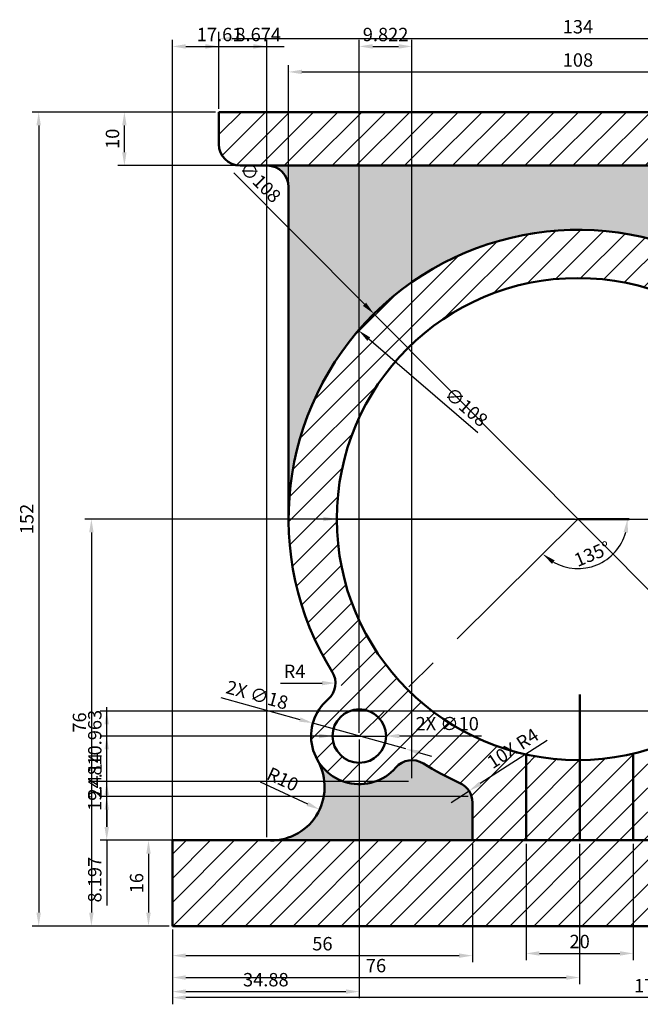
# Model space of a CAD drawing. Units: millimetres. Extents: x 2530 to 2750, y 1494 to 1677.
# Tile 1 of 2: x 2530 to 2646, y 1494 to 1677. Entities that reach past the tile are written whole.
import ezdxf

# ---------------------------------------------------------------- set-up
doc = ezdxf.new("R2010")
doc.units = ezdxf.units.MM
doc.linetypes.add('CENTER', pattern=[50.8, 31.75, -6.35, 6.35, -6.35])
for name, color, linetype, lineweight in [('M-CNTR', 1, 'CENTER', 18), ('M-DIMS', 2, 'Continuous', 25), ('M-HATC', 8, 'Continuous', 18), ('M-OUTL', 7, 'Continuous', 50)]:
    doc.layers.add(name, color=color, linetype=linetype, lineweight=lineweight)
doc.styles.get("Standard").update_dxf_attribs({"font": 'arial.ttf'})
doc.dimstyles.new('ISO-25', dxfattribs={"dimtxt": 2.5, "dimasz": 2.5, "dimexe": 1.25, "dimexo": 0.625, "dimtad": 1, "dimtxsty": 'Standard', "dimcen": 2.5, "dimadec": 0, "dimazin": 0, "dimtfac": 1, "dimtmove": 0, "dimatfit": 3, "dimfxl": 1, "dimarcsym": 0})

# ---------------------------------------------------------------- blocks, each defined once
blk = doc.blocks.new('*D1')
at = {"layer": 'Defpoints', "color": 0, "transparency": 16777216}
for p in [(2634.41, 1584.13), (2634.41, 1584.13), (2643.98, 1584.13), (2634.39, 1574.87), (2593.61, 1543.61)]:
    blk.add_point(p, dxfattribs=at)
at = {"layer": 'M-DIMS', "color": 0, "lineweight": -2, "transparency": 16777216}
blk.add_arc((2634.41, 1584.13), 9.26, 240.3168, 344.4892, dxfattribs=at)
at = {"layer": 'M-DIMS', "color": 0, "transparency": 16777216}
for points in [[(2642.92, 1581.71), (2643.75, 1581.6), (2643.67, 1584.13)], [(2629.57, 1575.75), (2630.07, 1576.41), (2627.84, 1577.6)]]:
    blk.add_solid(points, dxfattribs=at)
at = {"layer": 'M-DIMS', "color": 0, "transparency": 16777216, "insert": (2637.21, 1577.32), "char_height": 2.5, "attachment_point": 5, "rotation": 22.403}
blk.add_mtext('135°', dxfattribs=at)
blk = doc.blocks.new('*D2')
at = {"layer": 'Defpoints', "color": 0, "transparency": 16777216}
for p in [(2549.78, 1660.13), (2567.41, 1660.13), (2571.41, 1650.13)]:
    blk.add_point(p, dxfattribs=at)
at = {"layer": 'M-DIMS', "color": 0, "lineweight": -2, "transparency": 16777216}
for p, q in [((2566.78, 1660.13), (2548.53, 1660.13)), ((2549.78, 1652.63), (2549.78, 1657.63)), ((2570.78, 1650.13), (2548.53, 1650.13))]:
    blk.add_line(p, q, dxfattribs=at)
at = {"layer": 'M-DIMS', "color": 0, "transparency": 16777216}
for points in [[(2549.36, 1657.63), (2550.19, 1657.63), (2549.78, 1660.13)], [(2549.36, 1652.63), (2550.19, 1652.63), (2549.78, 1650.13)]]:
    blk.add_solid(points, dxfattribs=at)
at = {"layer": 'M-DIMS', "color": 0, "transparency": 16777216, "insert": (2547.88, 1655.13), "char_height": 2.5, "attachment_point": 5, "rotation": 90}
blk.add_mtext('10', dxfattribs=at)
blk = doc.blocks.new('*D3')
at = {"layer": 'Defpoints', "color": 0, "transparency": 16777216}
for p in [(2688.41, 1667.62), (2580.41, 1646.13), (2688.41, 1646.13)]:
    blk.add_point(p, dxfattribs=at)
at = {"layer": 'M-DIMS', "color": 0, "lineweight": -2, "transparency": 16777216}
for p, q in [((2580.41, 1646.75), (2580.41, 1668.87)), ((2688.41, 1646.75), (2688.41, 1668.87)), ((2582.91, 1667.62), (2685.91, 1667.62))]:
    blk.add_line(p, q, dxfattribs=at)
at = {"layer": 'M-DIMS', "color": 0, "transparency": 16777216}
for points in [[(2582.91, 1668.04), (2582.91, 1667.2), (2580.41, 1667.62)], [(2685.91, 1668.04), (2685.91, 1667.2), (2688.41, 1667.62)]]:
    blk.add_solid(points, dxfattribs=at)
at = {"layer": 'M-DIMS', "color": 0, "transparency": 16777216, "insert": (2634.41, 1669.52), "char_height": 2.5, "attachment_point": 5}
blk.add_mtext('108', dxfattribs=at)
blk = doc.blocks.new('*D4')
at = {"layer": 'Defpoints', "color": 0, "transparency": 16777216}
for p in [(2701.41, 1673.83), (2567.41, 1660.13), (2701.41, 1660.13)]:
    blk.add_point(p, dxfattribs=at)
at = {"layer": 'M-DIMS', "color": 0, "lineweight": -2, "transparency": 16777216}
for p, q in [((2567.41, 1660.75), (2567.41, 1675.08)), ((2701.41, 1660.75), (2701.41, 1675.08)), ((2569.91, 1673.83), (2698.91, 1673.83))]:
    blk.add_line(p, q, dxfattribs=at)
at = {"layer": 'M-DIMS', "color": 0, "transparency": 16777216}
for points in [[(2569.91, 1674.25), (2569.91, 1673.41), (2567.41, 1673.83)], [(2698.91, 1674.25), (2698.91, 1673.41), (2701.41, 1673.83)]]:
    blk.add_solid(points, dxfattribs=at)
at = {"layer": 'M-DIMS', "color": 0, "transparency": 16777216, "insert": (2634.41, 1675.73), "char_height": 2.5, "attachment_point": 5}
blk.add_mtext('134', dxfattribs=at)
blk = doc.blocks.new('*D5')
at = {"layer": 'Defpoints', "color": 0, "transparency": 16777216}
for p in [(2567.41, 1660.13), (2533.79, 1508.13), (2558.73, 1508.13)]:
    blk.add_point(p, dxfattribs=at)
at = {"layer": 'M-DIMS', "color": 0, "lineweight": -2, "transparency": 16777216}
for p, q in [((2566.78, 1660.13), (2532.54, 1660.13)), ((2533.79, 1657.63), (2533.79, 1510.63)), ((2558.11, 1508.13), (2532.54, 1508.13))]:
    blk.add_line(p, q, dxfattribs=at)
at = {"layer": 'M-DIMS', "color": 0, "transparency": 16777216}
for points in [[(2533.37, 1657.63), (2534.2, 1657.63), (2533.79, 1660.13)], [(2533.37, 1510.63), (2534.2, 1510.63), (2533.79, 1508.13)]]:
    blk.add_solid(points, dxfattribs=at)
at = {"layer": 'M-DIMS', "color": 0, "transparency": 16777216, "insert": (2531.89, 1584.13), "char_height": 2.5, "attachment_point": 5, "rotation": 90}
blk.add_mtext('152', dxfattribs=at)
blk = doc.blocks.new('*D6')
at = {"layer": 'Defpoints', "color": 0, "transparency": 16777216}
for p in [(2634.41, 1584.13), (2543.62, 1508.13), (2557.89, 1508.13)]:
    blk.add_point(p, dxfattribs=at)
at = {"layer": 'M-DIMS', "color": 0, "lineweight": -2, "transparency": 16777216}
for p, q in [((2633.78, 1584.13), (2542.37, 1584.13)), ((2543.62, 1581.63), (2543.62, 1510.63)), ((2557.27, 1508.13), (2542.37, 1508.13))]:
    blk.add_line(p, q, dxfattribs=at)
at = {"layer": 'M-DIMS', "color": 0, "transparency": 16777216}
for points in [[(2543.21, 1581.63), (2544.04, 1581.63), (2543.62, 1584.13)], [(2543.21, 1510.63), (2544.04, 1510.63), (2543.62, 1508.13)]]:
    blk.add_solid(points, dxfattribs=at)
at = {"layer": 'M-DIMS', "color": 0, "transparency": 16777216, "insert": (2541.72, 1546.13), "char_height": 2.5, "attachment_point": 5, "rotation": 90}
blk.add_mtext('76', dxfattribs=at)
blk = doc.blocks.new('*D7')
at = {"layer": 'Defpoints', "color": 0, "transparency": 16777216}
for p in [(2558.73, 1524.13), (2554.28, 1508.13), (2558.73, 1508.13)]:
    blk.add_point(p, dxfattribs=at)
at = {"layer": 'M-DIMS', "color": 0, "lineweight": -2, "transparency": 16777216}
for p, q in [((2558.11, 1524.13), (2553.03, 1524.13)), ((2554.28, 1521.63), (2554.28, 1510.63)), ((2558.11, 1508.13), (2553.03, 1508.13))]:
    blk.add_line(p, q, dxfattribs=at)
at = {"layer": 'M-DIMS', "color": 0, "transparency": 16777216}
for points in [[(2553.86, 1521.63), (2554.69, 1521.63), (2554.28, 1524.13)], [(2553.86, 1510.63), (2554.69, 1510.63), (2554.28, 1508.13)]]:
    blk.add_solid(points, dxfattribs=at)
at = {"layer": 'M-DIMS', "color": 0, "transparency": 16777216, "insert": (2552.38, 1516.13), "char_height": 2.5, "attachment_point": 5, "rotation": 90}
blk.add_mtext('16', dxfattribs=at)
blk = doc.blocks.new('*D8')
at = {"layer": 'Defpoints', "color": 0, "transparency": 16777216}
for p in [(2614.73, 1524.13), (2558.73, 1508.13), (2614.73, 1502.6)]:
    blk.add_point(p, dxfattribs=at)
at = {"layer": 'M-DIMS', "color": 0, "lineweight": -2, "transparency": 16777216}
for p, q in [((2614.73, 1523.5), (2614.73, 1501.35)), ((2558.73, 1507.5), (2558.73, 1501.35)), ((2561.23, 1502.6), (2612.23, 1502.6))]:
    blk.add_line(p, q, dxfattribs=at)
at = {"layer": 'M-DIMS', "color": 0, "transparency": 16777216}
for points in [[(2561.23, 1503.01), (2561.23, 1502.18), (2558.73, 1502.6)], [(2612.23, 1503.01), (2612.23, 1502.18), (2614.73, 1502.6)]]:
    blk.add_solid(points, dxfattribs=at)
at = {"layer": 'M-DIMS', "color": 0, "transparency": 16777216, "insert": (2586.73, 1504.5), "char_height": 2.5, "attachment_point": 5}
blk.add_mtext('56', dxfattribs=at)
blk = doc.blocks.new('*D9')
at = {"layer": 'Defpoints', "color": 0, "transparency": 16777216}
for p in [(2634.73, 1524.13), (2558.73, 1508.13), (2634.73, 1498.51)]:
    blk.add_point(p, dxfattribs=at)
at = {"layer": 'M-DIMS', "color": 0, "lineweight": -2, "transparency": 16777216}
for p, q in [((2634.73, 1523.5), (2634.73, 1497.26)), ((2558.73, 1507.5), (2558.73, 1497.26)), ((2561.23, 1498.51), (2632.23, 1498.51))]:
    blk.add_line(p, q, dxfattribs=at)
at = {"layer": 'M-DIMS', "color": 0, "transparency": 16777216}
for points in [[(2561.23, 1498.92), (2561.23, 1498.09), (2558.73, 1498.51)], [(2632.23, 1498.92), (2632.23, 1498.09), (2634.73, 1498.51)]]:
    blk.add_solid(points, dxfattribs=at)
at = {"layer": 'M-DIMS', "color": 0, "transparency": 16777216, "insert": (2596.73, 1500.41), "char_height": 2.5, "attachment_point": 5}
blk.add_mtext('76', dxfattribs=at)
blk = doc.blocks.new('*D10')
at = {"layer": 'Defpoints', "color": 0, "transparency": 16777216}
for p in [(2624.73, 1524.13), (2644.73, 1524.13), (2644.73, 1503.01)]:
    blk.add_point(p, dxfattribs=at)
at = {"layer": 'M-DIMS', "color": 0, "lineweight": -2, "transparency": 16777216}
for p, q in [((2624.73, 1523.5), (2624.73, 1501.76)), ((2644.73, 1523.5), (2644.73, 1501.76)), ((2627.23, 1503.01), (2642.23, 1503.01))]:
    blk.add_line(p, q, dxfattribs=at)
at = {"layer": 'M-DIMS', "color": 0, "transparency": 16777216}
for points in [[(2627.23, 1503.43), (2627.23, 1502.59), (2624.73, 1503.01)], [(2642.23, 1503.43), (2642.23, 1502.59), (2644.73, 1503.01)]]:
    blk.add_solid(points, dxfattribs=at)
at = {"layer": 'M-DIMS', "color": 0, "transparency": 16777216, "insert": (2634.73, 1504.91), "char_height": 2.5, "attachment_point": 5}
blk.add_mtext('20', dxfattribs=at)
blk = doc.blocks.new('*D14')
at = {"layer": 'Defpoints', "color": 0, "transparency": 16777216}
for p in [(2558.73, 1508.13), (2736.73, 1508.13), (2558.73, 1494.76)]:
    blk.add_point(p, dxfattribs=at)
at = {"layer": 'M-DIMS', "color": 0, "lineweight": -2, "transparency": 16777216}
for p, q in [((2558.73, 1507.5), (2558.73, 1493.51)), ((2736.73, 1507.5), (2736.73, 1493.51)), ((2734.23, 1494.76), (2561.23, 1494.76))]:
    blk.add_line(p, q, dxfattribs=at)
at = {"layer": 'M-DIMS', "color": 0, "transparency": 16777216}
for points in [[(2561.23, 1495.17), (2561.23, 1494.34), (2558.73, 1494.76)], [(2734.23, 1495.17), (2734.23, 1494.34), (2736.73, 1494.76)]]:
    blk.add_solid(points, dxfattribs=at)
at = {"layer": 'M-DIMS', "color": 0, "transparency": 16777216, "insert": (2647.73, 1496.66), "char_height": 2.5, "attachment_point": 5}
blk.add_mtext('178', dxfattribs=at)
blk = doc.blocks.new('*D17')
at = {"layer": 'Defpoints', "color": 0, "transparency": 16777216}
for p in [(2577.14, 1534.1), (2586.2, 1529.88)]:
    blk.add_point(p, dxfattribs=at)
at = {"layer": 'M-DIMS', "color": 0, "lineweight": -2, "transparency": 16777216}
blk.add_line((2575.13, 1535.03), (2583.94, 1530.94), dxfattribs=at)
at = {"layer": 'M-DIMS', "color": 0, "transparency": 16777216}
blk.add_solid([(2584.11, 1531.31), (2583.76, 1530.56), (2586.2, 1529.88)], dxfattribs=at)
at = {"layer": 'M-DIMS', "color": 0, "transparency": 16777216, "insert": (2579.2, 1535.24), "char_height": 2.5, "attachment_point": 5, "rotation": 335.0749}
blk.add_mtext('R10', dxfattribs=at)
blk = doc.blocks.new('*D24')
at = {"layer": 'Defpoints', "color": 0, "transparency": 16777216}
for p in [(2585.16, 1553.49), (2589.16, 1553.49)]:
    blk.add_point(p, dxfattribs=at)
at = {"layer": 'M-DIMS', "color": 0, "lineweight": -2, "transparency": 16777216}
blk.add_line((2578.89, 1553.49), (2586.66, 1553.49), dxfattribs=at)
at = {"layer": 'M-DIMS', "color": 0, "transparency": 16777216}
blk.add_solid([(2586.66, 1553.9), (2586.66, 1553.07), (2589.16, 1553.49)], dxfattribs=at)
at = {"layer": 'M-DIMS', "color": 0, "transparency": 16777216, "insert": (2581.53, 1555.36), "char_height": 2.5, "attachment_point": 5}
blk.add_mtext('R4', dxfattribs=at)
blk = doc.blocks.new('*D25')
at = {"layer": 'Defpoints', "color": 0, "transparency": 16777216}
for p in [(2672.67, 1607.82), (2596.15, 1560.44)]:
    blk.add_point(p, dxfattribs=at)
at = {"layer": 'M-DIMS', "color": 0, "lineweight": -2, "transparency": 16777216}
blk.add_line((2662, 1601.22), (2670.54, 1606.5), dxfattribs=at)
at = {"layer": 'M-DIMS', "color": 0, "transparency": 16777216}
blk.add_solid([(2670.32, 1606.86), (2670.76, 1606.15), (2672.67, 1607.82)], dxfattribs=at)
at = {"layer": 'M-DIMS', "color": 0, "transparency": 16777216, "insert": (2664.17, 1604.88), "char_height": 2.5, "attachment_point": 5, "rotation": 31.768}
blk.add_mtext('∅90', dxfattribs=at)
blk = doc.blocks.new('*D26')
at = {"layer": 'Defpoints', "color": 0, "transparency": 16777216}
for p in [(2593.48, 1619.36), (2675.33, 1548.9)]:
    blk.add_point(p, dxfattribs=at)
at = {"layer": 'M-DIMS', "color": 0, "lineweight": -2, "transparency": 16777216}
blk.add_line((2615.7, 1600.23), (2595.38, 1617.73), dxfattribs=at)
at = {"layer": 'M-DIMS', "color": 0, "transparency": 16777216}
blk.add_solid([(2595.65, 1618.04), (2595.11, 1617.41), (2593.48, 1619.36)], dxfattribs=at)
at = {"layer": 'M-DIMS', "color": 0, "transparency": 16777216, "insert": (2613.39, 1604.82), "char_height": 2.5, "attachment_point": 5, "rotation": 319.2753}
blk.add_mtext('∅108', dxfattribs=at)
blk = doc.blocks.new('*D27')
at = {"layer": 'Defpoints', "color": 0, "transparency": 16777216}
for p in [(2593.61, 1543.61), (2558.73, 1508.13), (2593.61, 1495.88)]:
    blk.add_point(p, dxfattribs=at)
at = {"layer": 'M-DIMS', "color": 0, "lineweight": -2, "transparency": 16777216}
for p, q in [((2593.61, 1542.98), (2593.61, 1494.63)), ((2558.73, 1507.5), (2558.73, 1494.63)), ((2561.23, 1495.88), (2591.11, 1495.88))]:
    blk.add_line(p, q, dxfattribs=at)
at = {"layer": 'M-DIMS', "color": 0, "transparency": 16777216}
for points in [[(2561.23, 1496.3), (2561.23, 1495.46), (2558.73, 1495.88)], [(2591.11, 1496.3), (2591.11, 1495.46), (2593.61, 1495.88)]]:
    blk.add_solid(points, dxfattribs=at)
at = {"layer": 'M-DIMS', "color": 0, "transparency": 16777216, "insert": (2576.17, 1497.78), "char_height": 2.5, "attachment_point": 5}
blk.add_mtext('34.88', dxfattribs=at)
blk = doc.blocks.new('*D28')
at = {"layer": 'Defpoints', "color": 0, "transparency": 16777216}
for p in [(2546.48, 1543.61), (2593.61, 1543.61), (2576.34, 1524.13)]:
    blk.add_point(p, dxfattribs=at)
at = {"layer": 'M-DIMS', "color": 0, "lineweight": -2, "transparency": 16777216}
for p, q in [((2592.99, 1543.61), (2545.23, 1543.61)), ((2546.48, 1526.63), (2546.48, 1541.11)), ((2575.72, 1524.13), (2545.23, 1524.13))]:
    blk.add_line(p, q, dxfattribs=at)
at = {"layer": 'M-DIMS', "color": 0, "transparency": 16777216}
for points in [[(2546.07, 1541.11), (2546.9, 1541.11), (2546.48, 1543.61)], [(2546.07, 1526.63), (2546.9, 1526.63), (2546.48, 1524.13)]]:
    blk.add_solid(points, dxfattribs=at)
at = {"layer": 'M-DIMS', "color": 0, "transparency": 16777216, "insert": (2544.58, 1533.87), "char_height": 2.5, "attachment_point": 5, "rotation": 90}
blk.add_mtext('19.48', dxfattribs=at)
blk = doc.blocks.new('*D31')
at = {"layer": 'Defpoints', "color": 0, "transparency": 16777216}
for p in [(2614.57, 1532.33), (2546.48, 1524.13), (2614.73, 1524.13)]:
    blk.add_point(p, dxfattribs=at)
at = {"layer": 'M-DIMS', "color": 0, "lineweight": -2, "transparency": 16777216}
for p, q in [((2613.94, 1532.33), (2545.23, 1532.33)), ((2546.48, 1529.83), (2546.48, 1526.63)), ((2614.11, 1524.13), (2545.23, 1524.13)), ((2546.48, 1524.13), (2546.48, 1511.94))]:
    blk.add_line(p, q, dxfattribs=at)
at = {"layer": 'M-DIMS', "color": 0, "transparency": 16777216}
for points in [[(2546.07, 1529.83), (2546.9, 1529.83), (2546.48, 1532.33)], [(2546.07, 1526.63), (2546.9, 1526.63), (2546.48, 1524.13)]]:
    blk.add_solid(points, dxfattribs=at)
at = {"layer": 'M-DIMS', "color": 0, "transparency": 16777216, "insert": (2544.58, 1516.78), "char_height": 2.5, "attachment_point": 5, "rotation": 90}
blk.add_mtext('8.197', dxfattribs=at)
blk = doc.blocks.new('*D32')
at = {"layer": 'Defpoints', "color": 0, "transparency": 16777216}
for p in [(2576.34, 1672.38), (2558.73, 1524.13), (2576.34, 1524.13)]:
    blk.add_point(p, dxfattribs=at)
at = {"layer": 'M-DIMS', "color": 0, "lineweight": -2, "transparency": 16777216}
for p, q in [((2558.73, 1524.75), (2558.73, 1673.63)), ((2576.34, 1524.75), (2576.34, 1673.63)), ((2561.23, 1672.38), (2573.84, 1672.38))]:
    blk.add_line(p, q, dxfattribs=at)
at = {"layer": 'M-DIMS', "color": 0, "transparency": 16777216}
for points in [[(2561.23, 1672.8), (2561.23, 1671.96), (2558.73, 1672.38)], [(2573.84, 1672.8), (2573.84, 1671.96), (2576.34, 1672.38)]]:
    blk.add_solid(points, dxfattribs=at)
at = {"layer": 'M-DIMS', "color": 0, "transparency": 16777216, "insert": (2567.54, 1674.28), "char_height": 2.5, "attachment_point": 5}
blk.add_mtext('17.61', dxfattribs=at)
blk = doc.blocks.new('*D33')
at = {"layer": 'Defpoints', "color": 0, "transparency": 16777216}
for p in [(2567.41, 1672.38), (2567.41, 1660.13), (2558.73, 1508.13)]:
    blk.add_point(p, dxfattribs=at)
at = {"layer": 'M-DIMS', "color": 0, "lineweight": -2, "transparency": 16777216}
for p, q in [((2558.73, 1508.75), (2558.73, 1673.63)), ((2567.41, 1660.75), (2567.41, 1673.63)), ((2561.23, 1672.38), (2564.91, 1672.38)), ((2567.41, 1672.38), (2579.59, 1672.38))]:
    blk.add_line(p, q, dxfattribs=at)
at = {"layer": 'M-DIMS', "color": 0, "transparency": 16777216}
for points in [[(2561.23, 1672.8), (2561.23, 1671.96), (2558.73, 1672.38)], [(2564.91, 1672.8), (2564.91, 1671.96), (2567.41, 1672.38)]]:
    blk.add_solid(points, dxfattribs=at)
at = {"layer": 'M-DIMS', "color": 0, "transparency": 16777216, "insert": (2574.75, 1674.28), "char_height": 2.5, "attachment_point": 5}
blk.add_mtext('8.674', dxfattribs=at)
blk = doc.blocks.new('*D36')
at = {"layer": 'Defpoints', "color": 0, "transparency": 16777216}
for p in [(2546.48, 1548.27), (2682.63, 1548.27), (2677.41, 1524.13)]:
    blk.add_point(p, dxfattribs=at)
at = {"layer": 'M-DIMS', "color": 0, "lineweight": -2, "transparency": 16777216}
for p, q in [((2682, 1548.27), (2545.23, 1548.27)), ((2546.48, 1526.63), (2546.48, 1545.77)), ((2676.78, 1524.13), (2545.23, 1524.13))]:
    blk.add_line(p, q, dxfattribs=at)
at = {"layer": 'M-DIMS', "color": 0, "transparency": 16777216}
for points in [[(2546.07, 1545.77), (2546.9, 1545.77), (2546.48, 1548.27)], [(2546.07, 1526.63), (2546.9, 1526.63), (2546.48, 1524.13)]]:
    blk.add_solid(points, dxfattribs=at)
at = {"layer": 'M-DIMS', "color": 0, "transparency": 16777216, "insert": (2544.6, 1536.2), "char_height": 2.5, "attachment_point": 5, "rotation": 90}
blk.add_mtext('24.14', dxfattribs=at)
blk = doc.blocks.new('*D37')
at = {"layer": 'Defpoints', "color": 0, "transparency": 16777216}
for p in [(2603.43, 1672.38), (2593.61, 1543.61), (2603.43, 1535.09)]:
    blk.add_point(p, dxfattribs=at)
at = {"layer": 'M-DIMS', "color": 0, "lineweight": -2, "transparency": 16777216}
for p, q in [((2593.61, 1544.23), (2593.61, 1673.63)), ((2603.43, 1535.72), (2603.43, 1673.63)), ((2596.11, 1672.38), (2600.93, 1672.38))]:
    blk.add_line(p, q, dxfattribs=at)
at = {"layer": 'M-DIMS', "color": 0, "transparency": 16777216}
for points in [[(2596.11, 1672.8), (2596.11, 1671.96), (2593.61, 1672.38)], [(2600.93, 1672.8), (2600.93, 1671.96), (2603.43, 1672.38)]]:
    blk.add_solid(points, dxfattribs=at)
at = {"layer": 'M-DIMS', "color": 0, "transparency": 16777216, "insert": (2598.52, 1674.28), "char_height": 2.5, "attachment_point": 5}
blk.add_mtext('9.822', dxfattribs=at)
blk = doc.blocks.new('*D38')
at = {"layer": 'Defpoints', "color": 0, "transparency": 16777216}
for p in [(2546.48, 1535.09), (2603.43, 1535.09), (2614.73, 1524.13)]:
    blk.add_point(p, dxfattribs=at)
at = {"layer": 'M-DIMS', "color": 0, "lineweight": -2, "transparency": 16777216}
for p, q in [((2546.48, 1535.09), (2546.48, 1548.99)), ((2602.81, 1535.09), (2545.23, 1535.09)), ((2546.48, 1526.63), (2546.48, 1532.59)), ((2614.11, 1524.13), (2545.23, 1524.13))]:
    blk.add_line(p, q, dxfattribs=at)
at = {"layer": 'M-DIMS', "color": 0, "transparency": 16777216}
for points in [[(2546.07, 1532.59), (2546.9, 1532.59), (2546.48, 1535.09)], [(2546.07, 1526.63), (2546.9, 1526.63), (2546.48, 1524.13)]]:
    blk.add_solid(points, dxfattribs=at)
at = {"layer": 'M-DIMS', "color": 0, "transparency": 16777216, "insert": (2544.58, 1543.29), "char_height": 2.5, "attachment_point": 5, "rotation": 90}
blk.add_mtext('10.963', dxfattribs=at)
blk = doc.blocks.new('*D39')
at = {"layer": 'Defpoints', "color": 0, "transparency": 16777216}
for p in [(2596.35, 1622.44), (2672.46, 1545.82)]:
    blk.add_point(p, dxfattribs=at)
at = {"layer": 'M-DIMS', "color": 0, "lineweight": -2, "transparency": 16777216}
for p, q in [((2570.17, 1648.8), (2594.59, 1624.22)), ((2672.46, 1545.82), (2596.35, 1622.44)), ((2674.22, 1544.04), (2675.99, 1542.27))]:
    blk.add_line(p, q, dxfattribs=at)
at = {"layer": 'M-DIMS', "color": 0, "transparency": 16777216}
for points in [[(2594.89, 1624.51), (2594.3, 1623.92), (2596.35, 1622.44)], [(2674.52, 1544.34), (2673.93, 1543.75), (2672.46, 1545.82)]]:
    blk.add_solid(points, dxfattribs=at)
at = {"layer": 'M-DIMS', "color": 0, "transparency": 16777216, "insert": (2574.92, 1646.82), "char_height": 2.5, "attachment_point": 5, "rotation": 314.806}
blk.add_mtext('∅108', dxfattribs=at)
blk = doc.blocks.new('*D40')
at = {"layer": 'Defpoints', "color": 0, "transparency": 16777216}
for p in [(2589.41, 1584.13), (2679.41, 1584.13)]:
    blk.add_point(p, dxfattribs=at)
at = {"layer": 'M-DIMS', "color": 0, "lineweight": -2, "transparency": 16777216}
for p, q in [((2586.91, 1584.13), (2584.41, 1584.13)), ((2589.41, 1584.13), (2679.41, 1584.13)), ((2710.18, 1584.13), (2681.91, 1584.13))]:
    blk.add_line(p, q, dxfattribs=at)
at = {"layer": 'M-DIMS', "color": 0, "transparency": 16777216}
for points in [[(2586.91, 1584.55), (2586.91, 1583.71), (2589.41, 1584.13)], [(2681.91, 1584.55), (2681.91, 1583.71), (2679.41, 1584.13)]]:
    blk.add_solid(points, dxfattribs=at)
at = {"layer": 'M-DIMS', "color": 0, "transparency": 16777216, "insert": (2706.41, 1586.1), "char_height": 2.5, "attachment_point": 5, "rotation": 0.0001}
blk.add_mtext('∅90', dxfattribs=at)
blk = doc.blocks.new('*D41')
at = {"layer": 'Defpoints', "color": 0, "transparency": 16777216}
for p in [(2584.94, 1546.02), (2602.28, 1541.2)]:
    blk.add_point(p, dxfattribs=at)
at = {"layer": 'M-DIMS', "color": 0, "lineweight": -2, "transparency": 16777216}
for p, q in [((2567.75, 1550.79), (2582.53, 1546.69)), ((2602.28, 1541.2), (2584.94, 1546.02)), ((2604.69, 1540.53), (2607.1, 1539.86))]:
    blk.add_line(p, q, dxfattribs=at)
at = {"layer": 'M-DIMS', "color": 0, "transparency": 16777216}
for points in [[(2582.64, 1547.09), (2582.42, 1546.28), (2584.94, 1546.02)], [(2604.8, 1540.93), (2604.58, 1540.13), (2602.28, 1541.2)]]:
    blk.add_solid(points, dxfattribs=at)
at = {"layer": 'M-DIMS', "color": 0, "transparency": 16777216, "insert": (2574.47, 1550.97), "char_height": 2.5, "attachment_point": 5, "rotation": 344.4794}
blk.add_mtext('2X ∅18', dxfattribs=at)
blk = doc.blocks.new('*D42')
at = {"layer": 'Defpoints', "color": 0, "transparency": 16777216}
for p in [(2588.61, 1543.61), (2598.61, 1543.61)]:
    blk.add_point(p, dxfattribs=at)
at = {"layer": 'M-DIMS', "color": 0, "lineweight": -2, "transparency": 16777216}
for p, q in [((2586.11, 1543.61), (2583.61, 1543.61)), ((2588.61, 1543.61), (2598.61, 1543.61)), ((2616.44, 1543.61), (2601.11, 1543.61))]:
    blk.add_line(p, q, dxfattribs=at)
at = {"layer": 'M-DIMS', "color": 0, "transparency": 16777216}
for points in [[(2586.11, 1544.03), (2586.11, 1543.19), (2588.61, 1543.61)], [(2601.11, 1544.02), (2601.11, 1543.19), (2598.61, 1543.61)]]:
    blk.add_solid(points, dxfattribs=at)
at = {"layer": 'M-DIMS', "color": 0, "transparency": 16777216, "insert": (2610.02, 1545.58), "char_height": 2.5, "attachment_point": 5, "rotation": 359.9972}
blk.add_mtext('2X ∅10', dxfattribs=at)
blk = doc.blocks.new('*D43')
at = {"layer": 'Defpoints', "color": 0, "transparency": 16777216}
for p in [(2614.09, 1533.36), (2610.73, 1531.18)]:
    blk.add_point(p, dxfattribs=at)
at = {"layer": 'M-DIMS', "color": 0, "lineweight": -2, "transparency": 16777216}
for p, q in [((2628.65, 1542.79), (2616.19, 1534.72)), ((2610.73, 1531.18), (2614.09, 1533.36))]:
    blk.add_line(p, q, dxfattribs=at)
at = {"layer": 'M-DIMS', "color": 0, "transparency": 16777216}
blk.add_solid([(2615.96, 1535.07), (2616.42, 1534.37), (2614.09, 1533.36)], dxfattribs=at)
at = {"layer": 'M-DIMS', "color": 0, "transparency": 16777216, "insert": (2622.43, 1541.03), "char_height": 2.5, "attachment_point": 5, "rotation": 32.9488}
blk.add_mtext('10X R4', dxfattribs=at)

msp = doc.modelspace()

# ---------------------------------------------------------------- hatches: boundary and pattern name
at = {"layer": 'M-HATC'}
h = msp.add_hatch(dxfattribs=at)
h.set_pattern_fill('ANSI31', color=256)
h.paths.add_polyline_path([(2701.4085, 1660.1289), (2688.4085, 1660.1289), (2567.4085, 1660.1289), (2567.4085, 1654.1289, 0.41421356), (2571.4085, 1650.1289), (2580.4085, 1650.1289), (2688.4085, 1650.1289), (2697.4085, 1650.1289, 0.41421356), (2701.4085, 1654.1289)])
h.paths.add_polyline_path([(2679.4085, 1584.1289, -0.34791599), (2644.7344, 1540.3297), (2644.7344, 1524.1289), (2654.7344, 1524.1289), (2658.7344, 1524.1289, -0.41421356), (2654.7344, 1528.1289), (2654.7344, 1531.4768, -0.29243225), (2657.0568, 1535.108, 0.47416598), (2677.944, 1616.0767, 1.63457651), (2666.6504, 1627.447, 0.86114512), (2590.873, 1552.1812, 1.31927608), (2600.4123, 1537.7124, -0.37066508), (2605.5707, 1538.4739, 0.03574325), (2612.3671, 1534.8321, -0.29578567), (2614.7344, 1531.1805), (2614.7344, 1524.1289), (2624.7344, 1524.1289), (2624.7344, 1540.1811, -0.14401207), (2602.4811, 1552.4171), (2597.1599, 1547.1318, -0.19803221), (2598.6124, 1543.6082, -1), (2588.6124, 1543.6082, -0.6694042), (2597.1599, 1547.1318), (2602.4811, 1552.4171, -0.19803221), (2589.4085, 1584.1289, -1)])
h.paths.add_polyline_path([(2680.2046, 1624.6496, -1), (2670.2046, 1624.6496, -1)], flags=16)
h.paths.add_polyline_path([(2736.7344, 1524.1289), (2735.977, 1524.1289, -0.04128859), (2734.3283, 1524.1289), (2577.9283, 1524.1289, -0.03968429), (2576.3434, 1524.1289), (2558.7344, 1524.1289), (2558.7344, 1508.1289), (2736.7344, 1508.1289)])
h = msp.add_hatch(color=256, dxfattribs=at)
h.dxf.hatch_style = 1
h.paths.add_polyline_path([(2688.4085, 1646.1289, -0.41421356), (2692.4085, 1650.1289), (2688.4085, 1650.1289), (2580.4085, 1650.1289), (2576.4085, 1650.1289, -0.41421356), (2580.4085, 1646.1289), (2580.4085, 1584.1289, -0.61677219), (2666.6504, 1627.447, -1.63457651), (2677.944, 1616.0767, -0.15960296), (2688.4085, 1584.1289)])
h.paths.add_polyline_path([(2696.1494, 1571.5708, -0.30814487), (2688.4024, 1583.3173, -0.28835772), (2657.0568, 1535.108, 0.29243225), (2654.7344, 1531.4768), (2654.7344, 1528.1289, 0.41421356), (2658.7344, 1524.1289), (2677.4085, 1524.1289), (2682.6254, 1548.2693, -0.35316368), (2694.8434, 1558.1289), (2696.2102, 1558.1289)])
h.paths.add_polyline_path([(2713.9085, 1558.1289, 0.30415201), (2706.158, 1569.6915), (2706.2106, 1558.0572, -0.18754445), (2709.4561, 1551.5776), (2714.9622, 1524.1289), (2734.3283, 1524.1289, -0.27714511), (2725.9689, 1530.1379)])
h.paths.add_polyline_path([(2614.7344, 1531.1805, 0.29578567), (2612.3671, 1534.8321, -0.03574325), (2605.5707, 1538.4739, 0.37066508), (2600.4123, 1537.7124, -0.512533), (2585.8599, 1539.0368), (2585.8445, 1539.0127, -0.54802528), (2577.9283, 1524.1289), (2614.7344, 1524.1289)])
h = msp.add_hatch(dxfattribs=at)
h.set_pattern_fill('ANSI31', color=256)
h.paths.add_polyline_path([(2634.7344, 1539.1301, -0.05603695), (2624.7344, 1540.1811), (2624.7344, 1524.1289), (2634.7344, 1524.1289)])
h.paths.add_polyline_path([(2644.7344, 1540.3297, -0.05613012), (2634.7344, 1539.1301), (2634.7344, 1524.1289), (2644.7344, 1524.1289)])

# ---------------------------------------------------------------- linework, layer by layer
at = {"layer": 'M-CNTR'}
msp.add_line((2634.4085, 1584.1289), (2593.6124, 1543.6082), dxfattribs=at)
at = {"layer": 'M-OUTL'}
for p, q in [((2567.4085, 1654.1289), (2567.4085, 1660.1289)), ((2567.4085, 1660.1289), (2688.4085, 1660.1289)), ((2580.4085, 1650.1289), (2571.4085, 1650.1289)), ((2580.4085, 1650.1289), (2688.4085, 1650.1289)), ((2580.4085, 1584.1289), (2580.4085, 1646.1289)), ((2634.4085, 1584.1289), (2643.9827, 1584.1289)), ((2634.7344, 1524.1289), (2634.7344, 1551.3374)), ((2585.8445, 1539.0127), (2585.8599, 1539.0368)), ((2590.5939, 1540.6102), (2590.5939, 1540.6102)), ((2624.7344, 1524.1289), (2624.7344, 1540.1811)), ((2644.7344, 1524.1289), (2644.7344, 1540.3297)), ((2614.7344, 1524.1289), (2614.7344, 1531.1805)), ((2558.7344, 1524.1289), (2736.7344, 1524.1289)), ((2558.7344, 1524.1289), (2614.7344, 1524.1289)), ((2558.7344, 1508.1289), (2558.7344, 1524.1289)), ((2614.7344, 1524.1289), (2634.7344, 1524.1289)), ((2644.7344, 1524.1289), (2654.7344, 1524.1289)), ((2558.7344, 1508.1289), (2736.7344, 1508.1289))]:
    msp.add_line(p, q, dxfattribs=at)
for centre, radius in [((2634.4085, 1584.1289), 45), ((2593.6124, 1543.6082), 5)]:
    msp.add_circle(centre, radius, dxfattribs=at)
for centre, radius, start, end in [((2571.4085, 1654.1289), 4, 180, 270), ((2576.4085, 1646.1289), 4, 0, 90), ((2634.4085, 1584.1289), 54, 57.721584, 211.89027), ((2585.1629, 1553.4879), 4, 310.538333, 31.89027), ((2593.6124, 1543.6082), 9, 130.538333, 319.073521), ((2577.1358, 1534.0975), 10, 265.4549, 29.440521), ((2603.4345, 1535.0921), 4, 57.721584, 139.073521), ((2634.4085, 1584.1289), 54, 237.721584, 245.909848), ((2610.7344, 1531.1805), 4, 360, 65.909848)]:
    msp.add_arc(centre, radius, start, end, dxfattribs=at)

# ---------------------------------------------------------------- dimensions: what is measured, and where the dimension line sits
at = {"layer": 'M-DIMS'}
for base, p1, p2, override, picture, middle in [((2701.4085, 1673.8298), (2567.4085, 1660.1289), (2701.4085, 1660.1289), {"dimclrd": 0, "dimclre": 0, "dimclrt": 0}, '*D4', (2634.4085, 1675.7321)), ((2576.3434, 1672.3789), (2558.7344, 1524.1289), (2576.3434, 1524.1289), {"dimdec": 2, "dimlfac": 1, "dimrnd": 0, "dimzin": 0, "dimdsep": 46, "dimlunit": 2}, '*D32', (2567.5389, 1674.2804)), ((2567.4085, 1672.3789), (2558.7344, 1508.1289), (2567.4085, 1660.1289), {"dimdec": 3, "dimlfac": 1, "dimrnd": 0, "dimzin": 0, "dimdsep": 46, "dimlunit": 2}, '*D33', (2574.7482, 1674.2804)), ((2603.4345, 1672.3789), (2593.6124, 1543.6082), (2603.4345, 1535.0921), {"dimdec": 3, "dimlfac": 1, "dimrnd": 0, "dimzin": 0, "dimdsep": 46, "dimlunit": 2}, '*D37', (2598.5235, 1674.2804)), ((2688.4085, 1667.6183), (2580.4085, 1646.1289), (2688.4085, 1646.1289), {"dimclrd": 0, "dimclre": 0, "dimclrt": 0}, '*D3', (2634.4085, 1669.5198)), ((2593.6124, 1495.8789), (2558.7344, 1508.1289), (2593.6124, 1543.6082), {"dimdec": 2, "dimlfac": 1, "dimrnd": 0, "dimzin": 0, "dimdsep": 46, "dimlunit": 2}, '*D27', (2576.1734, 1497.7812)), ((2614.7344, 1502.595), (2558.7344, 1508.1289), (2614.7344, 1524.1289), {"dimclrd": 0, "dimclre": 0, "dimclrt": 0}, '*D8', (2586.7344, 1504.4964)), ((2634.7344, 1498.5081), (2558.7344, 1508.1289), (2634.7344, 1524.1289), {"dimclrd": 0, "dimclre": 0, "dimclrt": 0}, '*D9', (2596.7344, 1500.4096)), ((2644.7344, 1503.0087), (2624.7344, 1524.1289), (2644.7344, 1524.1289), {"dimclrd": 0, "dimclre": 0, "dimclrt": 0}, '*D10', (2634.7344, 1504.9102)), ((2558.7344, 1494.7581), (2736.7344, 1508.1289), (2558.7344, 1508.1289), {"dimclrd": 0, "dimclre": 0, "dimclrt": 0}, '*D14', (2647.7344, 1496.6596))]:
    dim = msp.add_linear_dim(base=base, p1=p1, p2=p2, dimstyle='ISO-25', override=override, dxfattribs=at)
    dim.commit()
    dim.dimension.update_dxf_attribs({"geometry": picture, "text_midpoint": middle})
for base, p1, p2, override, picture, middle in [((2533.787, 1508.1289), (2567.4085, 1660.1289), (2558.7344, 1508.1289), {"dimclrd": 0, "dimclre": 0, "dimclrt": 0}, '*D5', (2531.8856, 1584.1289)), ((2549.7773, 1660.1289), (2571.4085, 1650.1289), (2567.4085, 1660.1289), {"dimclrd": 0, "dimclre": 0, "dimclrt": 0}, '*D2', (2547.8759, 1655.1289)), ((2543.6222, 1508.1289), (2634.4085, 1584.1289), (2557.8919, 1508.1289), {"dimclrd": 0, "dimclre": 0, "dimclrt": 0}, '*D6', (2541.7208, 1546.1289)), ((2546.4844, 1535.0921), (2614.7344, 1524.1289), (2603.4345, 1535.0921), {"dimdec": 3, "dimlfac": 1, "dimrnd": 0, "dimzin": 0, "dimdsep": 46, "dimlunit": 2}, '*D38', (2544.5822, 1543.2887)), ((2546.4844, 1548.2693), (2677.4085, 1524.1289), (2682.6254, 1548.2693), {"dimdec": 2, "dimlfac": 1, "dimrnd": 0, "dimzin": 0, "dimdsep": 46, "dimlunit": 2}, '*D36', (2544.6043, 1536.1991)), ((2546.4844, 1543.6082), (2576.3434, 1524.1289), (2593.6124, 1543.6082), {"dimdec": 2, "dimlfac": 1, "dimrnd": 0, "dimzin": 0, "dimdsep": 46, "dimlunit": 2}, '*D28', (2544.583, 1533.8686)), ((2546.4844, 1524.1289), (2614.5671, 1532.326), (2614.7344, 1524.1289), {"dimdec": 3, "dimlfac": 1, "dimrnd": 0, "dimzin": 0, "dimdsep": 46, "dimlunit": 2}, '*D31', (2544.583, 1516.7841)), ((2554.277, 1508.1289), (2558.7344, 1524.1289), (2558.7344, 1508.1289), {"dimclrd": 0, "dimclre": 0, "dimclrt": 0}, '*D7', (2552.3755, 1516.1289))]:
    dim = msp.add_linear_dim(base=base, p1=p1, p2=p2, angle=90, dimstyle='ISO-25', override=override, dxfattribs=at)
    dim.commit()
    dim.dimension.update_dxf_attribs({"geometry": picture, "text_midpoint": middle})
for p1, p2, override, picture, middle in [((2672.4628, 1545.8161), (2596.3542, 1622.4418), {"dimdec": 0, "dimlfac": 1, "dimrnd": 0, "dimzin": 0, "dimdsep": 46, "dimlunit": 2}, '*D39', (2573.5217, 1645.4295)), ((2675.3326, 1548.898), (2593.4844, 1619.3599), {"dimclrd": 0, "dimclre": 0, "dimclrt": 0}, '*D26', (2612.1037, 1603.3308)), ((2596.1501, 1560.4373), (2672.6669, 1607.8206), {"dimclrd": 0, "dimclre": 0, "dimclrt": 0}, '*D25', (2665.2096, 1603.2027)), ((2589.4085, 1584.1289), (2679.4085, 1584.129), {"dimdec": 0, "dimlfac": 1, "dimrnd": 0, "dimzin": 0, "dimdsep": 46, "dimlunit": 2}, '*D40', (2706.4085, 1584.129))]:
    dim = msp.add_diameter_dim_2p(p1=p1, p2=p2, dimstyle='ISO-25', override=override, dxfattribs=at)
    dim.commit()
    dim.dimension.update_dxf_attribs({"geometry": picture, "text_midpoint": middle, "dimtype": 163})
dim = msp.add_angular_dim_2l(base=(2634.3876, 1574.8659), line1=((2634.4085, 1584.1289), (2643.9827, 1584.1289)), line2=((2634.4085, 1584.1289), (2593.6124, 1543.6082)), dimstyle='ISO-25', override={"dimclrd": 0, "dimclre": 0, "dimclrt": 0}, dxfattribs=at)
dim.commit()
dim.dimension.update_dxf_attribs({"geometry": '*D1', "text_midpoint": (2637.2138, 1577.3237)})
for p1, p2, picture, middle in [((2602.2842, 1541.2), (2584.9406, 1546.0165), '*D41', (2573.9381, 1549.072)), ((2588.6124, 1543.6085), (2598.6124, 1543.608), '*D42', (2610.0244, 1543.6074))]:
    dim = msp.add_diameter_dim_2p(p1=p1, p2=p2, text='2X <>', dimstyle='ISO-25', override={"dimdec": 0, "dimlfac": 1, "dimrnd": 0, "dimzin": 0, "dimdsep": 46, "dimlunit": 2}, dxfattribs=at)
    dim.commit()
    dim.dimension.update_dxf_attribs({"geometry": picture, "text_midpoint": middle})
for center, mpoint, picture, middle in [((2585.1629, 1553.4879), (2589.1629, 1553.4879), '*D24', (2581.5274, 1553.4879)), ((2577.1358, 1534.0975), (2586.2044, 1529.8832), '*D17', (2578.3985, 1533.5107))]:
    dim = msp.add_radius_dim(center=center, mpoint=mpoint, dimstyle='ISO-25', override={"dimclrd": 0, "dimclre": 0, "dimclrt": 0}, dxfattribs=at)
    dim.commit()
    dim.dimension.update_dxf_attribs({"geometry": picture, "text_midpoint": middle, "dimtype": 164})
dim = msp.add_radius_dim(center=(2610.7344, 1531.1805), mpoint=(2614.0911, 1533.356), text='10X <>', dimstyle='ISO-25', override={"dimdec": 0, "dimlfac": 1, "dimrnd": 0, "dimzin": 0, "dimdsep": 46, "dimlunit": 2}, dxfattribs=at)
dim.commit()
dim.dimension.update_dxf_attribs({"geometry": '*D43', "text_midpoint": (2622.4344, 1541.0296)})

doc.saveas('drawing.dxf')
